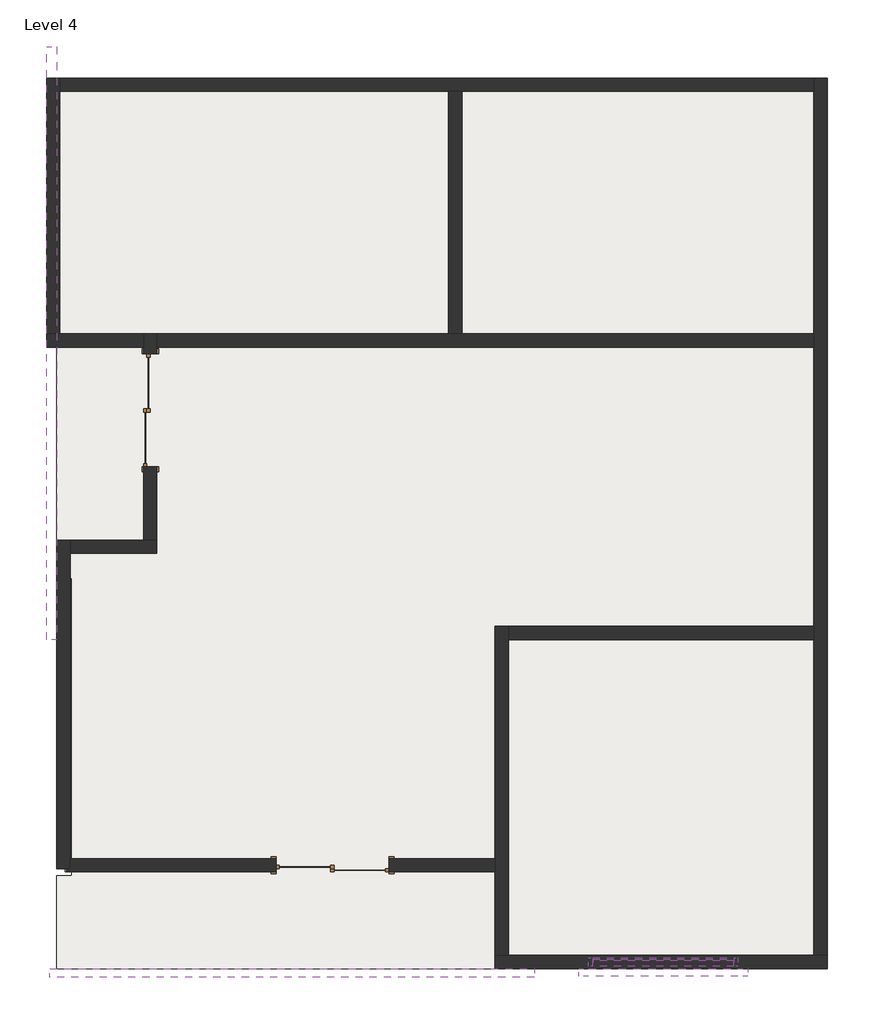
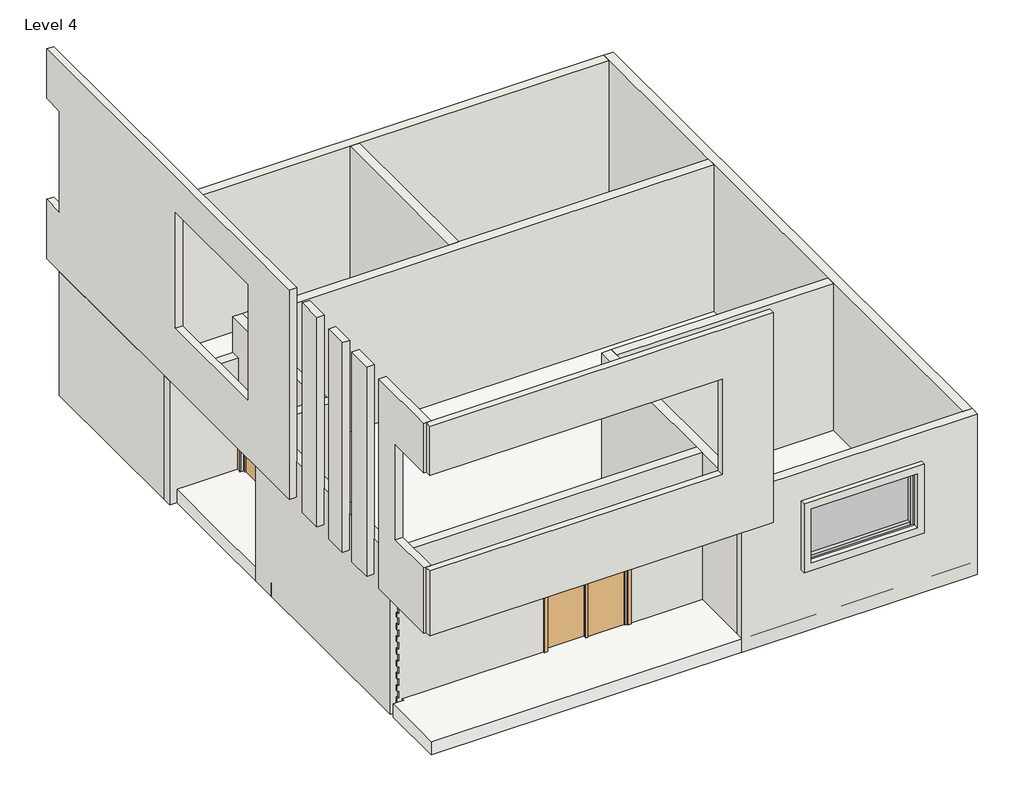
# One storey: 16 walls, 4 members, 2 doors, 1 plate, 1 roof.
"""IFC4 building model written with IfcOpenShell, lengths in millimetres."""

from ifc_helpers import new_model, si_unit, frame, origin, place, context, project, spatial, polyline, outline, extrude, faceted_brep, transform, mapped, element, save
from components import door_076b30e0, member_3a6679d5, member_c08f7e50, system_panel_glazed_5a0db22b, walls_2_walls_1_3aef9765, walls_7_walls_7_28da2d4c, walls_8_walls_8_57d20523

model = new_model("IFC4")

# Units and contexts
model_context = context("Model", 3, world=origin())
ifc_project = project(units=[si_unit("LENGTHUNIT", "METRE", prefix="MILLI")], contexts=[model_context])

# Site, building, storey
site = spatial("IfcSite", under=ifc_project)
building = spatial("IfcBuilding", under=site)
storey = spatial("IfcBuildingStorey", under=building, Name="Level 4", Elevation=10972.8)

# Doors
placement = place(None, origin())
door_shape = door_076b30e0(model_context)
element("IfcDoor", 1, ObjectType="Door-Double-Sliding : 68\" x 80\"", at=placement, inside=storey, context=model_context, shape_type="MappedRepresentation", body=[
    mapped(door_shape, transform((-7304.8227738, 4545.1674246, 11074.4), x_axis=(0.0, 1.0, 0.0), y_axis=(-1.0, 0.0, 0.0), z_axis=(0.0, 0.0, 1.0))),
])
element("IfcDoor", 2, ObjectType="Door-Double-Sliding : 68\" x 80\"", at=placement, inside=storey, context=model_context, shape_type="MappedRepresentation", body=[
    mapped(door_shape, transform((-4644.5436544, -2281.0825754, 11176.0), x_axis=(-1.0, 0.0, 0.0), y_axis=(0.0, -1.0, 0.0), z_axis=(0.0, 0.0, 1.0))),
])

# Members
member_shape = member_3a6679d5(model_context)
element("IfcMember", 3, ObjectType="Rectangular Mullion : 2.5\" x 5\" rectangular", at=placement, inside=storey, context=model_context, shape_type="MappedRepresentation", body=[
    mapped(member_shape, transform((1560.0533085, -3887.6325754, 12576.3422066), x_axis=(1.0, 0.0, 0.0), y_axis=(0.0, -1.0, 0.0), z_axis=(0.0, 0.0, -1.0))),
])
member_2_shape = member_c08f7e50(model_context)
element("IfcMember", 4, ObjectType="Rectangular Mullion : 2.5\" x 5\" rectangular", at=placement, inside=storey, context=model_context, shape_type="MappedRepresentation", body=[
    mapped(member_2_shape, transform((-662.4466915, -3887.6325754, 12576.3422066), x_axis=(0.0, 0.0, -1.0), y_axis=(0.0, -1.0, 0.0), z_axis=(-1.0, 0.0, 0.0))),
])
element("IfcMember", 5, ObjectType="Rectangular Mullion : 2.5\" x 5\" rectangular", at=placement, inside=storey, context=model_context, shape_type="MappedRepresentation", body=[
    mapped(member_2_shape, transform((1496.5533085, -3887.6325754, 13807.224337), x_axis=(0.0, 0.0, 1.0), y_axis=(0.0, -1.0, 0.0), z_axis=(1.0, 0.0, 0.0))),
])
element("IfcMember", 6, ObjectType="Rectangular Mullion : 2.5\" x 5\" rectangular", at=placement, inside=storey, context=model_context, shape_type="MappedRepresentation", body=[
    mapped(member_shape, transform((-725.9466915, -3887.6325754, 13807.224337), x_axis=(-1.0, 0.0, 0.0), y_axis=(0.0, -1.0, 0.0), z_axis=(0.0, 0.0, 1.0))),
])

# Plate
system_panel_glazed_shape = system_panel_glazed_5a0db22b(model_context)
element("IfcPlate", 7, ObjectType="System Panel : Glazed", at=placement, inside=storey, context=model_context, shape_type="MappedRepresentation", body=[
    mapped(system_panel_glazed_shape, transform((417.0533085, -3887.6325754, 12639.8422066), x_axis=(1.0, 0.0, 0.0), y_axis=(0.0, 1.0, 0.0), z_axis=(0.0, 0.0, 1.0))),
])

# Roof
element("IfcRoof", 8, ObjectType="Generic - 12\"", at=placement, inside=storey, context=model_context, shape_type="SweptSolid", body=[
    extrude(outline(polyline([(-8860.5727738, 9472.7674246), (2924.6563456, 9472.7674246), (2924.6563456, -3989.2325754), (-8860.5727738, -3989.2325754), (-8860.5727738, -2566.8325754), (-8631.9727738, -2566.8325754), (-8631.9727738, 1979.7674246), (-8860.5727738, 1979.7674246), (-8860.5727738, 9472.7674246)])), frame((0.0, 0.0, 10972.8), z_axis=(0.0, 0.0, 1.0), x_axis=(1.0, 0.0, 0.0)), (0.0, 0.0, 1.0), 304.8),
])

# Walls
element("IfcWall", 9, ObjectType="Generic - 8\"", at=placement, inside=storey, context=model_context, shape_type="Brep", body=[
    faceted_brep([(2924.6563456, -3786.0325754, 10972.8), (2721.4563456, -3786.0325754, 10972.8), (-1952.1436544, -3786.0325754, 10972.8), (-2155.3436544, -3786.0325754, 10972.8), (-2155.3436544, -3786.0325754, 14630.4), (-1952.1436544, -3786.0325754, 14630.4), (2721.4563456, -3786.0325754, 14630.4), (2924.6563456, -3786.0325754, 14630.4), (1560.0533085, -3786.0325754, 13807.224337), (-725.9466915, -3786.0325754, 13807.224337), (-725.9466915, -3786.0325754, 12576.3422066), (1560.0533085, -3786.0325754, 12576.3422066), (2924.6563456, -3989.2325754, 10972.8), (2924.6563456, -3989.2325754, 14630.4), (-2155.3436544, -3989.2325754, 14630.4), (-2155.3436544, -3989.2325754, 10972.8), (1560.0533085, -3989.2325754, 13807.224337), (1560.0533085, -3989.2325754, 12576.3422066), (-725.9466915, -3989.2325754, 12576.3422066), (-725.9466915, -3989.2325754, 13807.224337)], [[[0, 1, 2, 3, 4, 5, 6, 7], [8, 9, 10, 11]], [[12, 13, 14, 15], [16, 17, 18, 19]], [[4, 3, 15, 14]], [[0, 7, 13, 12]], [[3, 2, 1, 0, 12, 15]], [[7, 6, 5, 4, 14, 13]], [[9, 8, 16, 19]], [[10, 9, 19, 18]], [[11, 10, 18, 17]], [[8, 11, 17, 16]]]),
])
element("IfcWall", 10, ObjectType="Generic - 8\"", at=placement, inside=storey, context=model_context, shape_type="Brep", body=[
    faceted_brep([(-1952.1436544, -3786.0325754, 10972.8), (-1952.1436544, 1039.9674246, 10972.8), (-1952.1436544, 1243.1674246, 10972.8), (-1952.1436544, 1243.1674246, 14630.4), (-1952.1436544, 1039.9674246, 14630.4), (-1952.1436544, -3786.0325754, 14630.4), (-2155.3436544, -3786.0325754, 10972.8), (-2155.3436544, -3786.0325754, 14630.4), (-2155.3436544, -2509.6825754, 14630.4), (-2155.3436544, -2306.4825754, 14630.4), (-2155.3436544, 1243.1674246, 14630.4), (-2155.3436544, 1243.1674246, 10972.8), (-2155.3436544, -2306.4825754, 10972.8), (-2155.3436544, -2509.6825754, 10972.8)], [[[0, 1, 2, 3, 4, 5]], [[6, 7, 8, 9, 10, 11, 12, 13]], [[2, 1, 0, 6, 13, 12, 11]], [[5, 4, 3, 10, 9, 8, 7]], [[0, 5, 7, 6]], [[3, 2, 11, 10]]]),
])
element("IfcWall", 11, ObjectType="Generic - 8\"", at=placement, inside=storey, context=model_context, shape_type="SweptSolid", body=[
    extrude(outline(polyline([(2716.475018, 1039.9674246), (-1952.1436544, 1039.9674246), (-1952.1436544, 1243.1674246), (2716.475018, 1243.1674246), (2716.475018, 1039.9674246)])), frame((0.0, 0.0, 10972.8), z_axis=(0.0, 0.0, 1.0), x_axis=(1.0, 0.0, 0.0)), (0.0, 0.0, 1.0), 3657.6),
])
element("IfcWall", 12, ObjectType="Generic - 8\"", at=placement, inside=storey, context=model_context, shape_type="SweptSolid", body=[
    extrude(outline(polyline([(2924.6563456, 9625.1674246), (2924.6563456, -3786.0325754), (2721.4563456, -3786.0325754), (2721.4563456, 9625.1674246), (2924.6563456, 9625.1674246)])), frame((0.0, 0.0, 10972.8), z_axis=(0.0, 0.0, 1.0), x_axis=(1.0, 0.0, 0.0)), (0.0, 0.0, 1.0), 3657.6),
])
element("IfcWall", 13, ObjectType="Generic - 8\"", at=placement, inside=storey, context=model_context, shape_type="Brep", body=[
    faceted_brep([(-8657.3727738, -2465.2325754, 10972.8), (-8657.3727738, -2306.4825754, 10972.8), (-8657.3727738, 2360.7674246, 10972.8), (-8657.3727738, 2563.9674246, 10972.8), (-8657.3727738, 2563.9674246, 14630.4), (-8657.3727738, 2360.7674246, 14630.4), (-8657.3727738, -2306.4825754, 14630.4), (-8657.3727738, -2465.2325754, 14630.4), (-8860.5727738, -2465.2325754, 10972.8), (-8860.5727738, -2465.2325754, 11328.4), (-8860.5727738, -2465.2325754, 11480.8), (-8860.5727738, -2465.2325754, 11607.8), (-8860.5727738, -2465.2325754, 11760.2), (-8860.5727738, -2465.2325754, 11887.2), (-8860.5727738, -2465.2325754, 12039.6), (-8860.5727738, -2465.2325754, 12166.6), (-8860.5727738, -2465.2325754, 12319.0), (-8860.5727738, -2465.2325754, 12446.0), (-8860.5727738, -2465.2325754, 12598.4), (-8860.5727738, -2465.2325754, 12725.4), (-8860.5727738, -2465.2325754, 12877.8), (-8860.5727738, -2465.2325754, 13004.8), (-8860.5727738, -2465.2325754, 13157.2), (-8860.5727738, -2465.2325754, 13258.8), (-8860.5727738, -2465.2325754, 13411.2), (-8860.5727738, -2465.2325754, 13563.6), (-8860.5727738, -2465.2325754, 13716.0), (-8860.5727738, -2465.2325754, 14630.4), (-8860.5727738, 2563.9674246, 14630.4), (-8860.5727738, 2563.9674246, 10972.8), (-8733.5727738, -2465.2325754, 10972.8), (-8733.5727738, -2465.2325754, 14630.4)], [[[0, 1, 2, 3, 4, 5, 6, 7]], [[8, 9, 10, 11, 12, 13, 14, 15, 16, 17, 18, 19, 20, 21, 22, 23, 24, 25, 26, 27, 28, 29]], [[3, 2, 1, 0, 30, 8, 29]], [[7, 6, 5, 4, 28, 27, 31]], [[0, 7, 31, 27, 26, 25, 24, 23, 22, 21, 20, 19, 18, 17, 16, 15, 14, 13, 12, 11, 10, 9, 8, 30]], [[4, 3, 29, 28]]]),
])
element("IfcWall", 14, ObjectType="Generic - 8\"", at=placement, inside=storey, context=model_context, shape_type="Brep", body=[
    faceted_brep([(-8657.3727738, 2360.7674246, 10972.8), (-7330.2227738, 2360.7674246, 10972.8), (-7330.2227738, 2360.7674246, 14630.4), (-8657.3727738, 2360.7674246, 14630.4), (-8657.3727738, 2563.9674246, 10972.8), (-8657.3727738, 2563.9674246, 14630.4), (-7533.4227738, 2563.9674246, 14630.4), (-7330.2227738, 2563.9674246, 14630.4), (-7330.2227738, 2563.9674246, 10972.8), (-7533.4227738, 2563.9674246, 10972.8)], [[[0, 1, 2, 3]], [[4, 5, 6, 7, 8, 9]], [[1, 0, 4, 9, 8]], [[3, 2, 7, 6, 5]], [[0, 3, 5, 4]], [[2, 1, 8, 7]]]),
])
element("IfcWall", 15, ObjectType="Generic - 8\"", at=placement, inside=storey, context=model_context, shape_type="Brep", body=[
    faceted_brep([(-7330.2227738, 2563.9674246, 10972.8), (-7330.2227738, 5510.3674246, 10972.8), (-7330.2227738, 5713.5674246, 10972.8), (-7330.2227738, 5713.5674246, 14630.4), (-7330.2227738, 5510.3674246, 14630.4), (-7330.2227738, 2563.9674246, 14630.4), (-7330.2227738, 3681.5674246, 13106.4), (-7330.2227738, 5408.7674246, 13106.4), (-7330.2227738, 5408.7674246, 11074.4), (-7330.2227738, 3681.5674246, 11074.4), (-7533.4227738, 2563.9674246, 10972.8), (-7533.4227738, 2563.9674246, 14630.4), (-7533.4227738, 5713.5674246, 14630.4), (-7533.4227738, 5713.5674246, 13807.224337), (-7533.4227738, 5713.5674246, 10972.8), (-7533.4227738, 5510.3674246, 10972.8), (-7533.4227738, 3681.5674246, 13106.4), (-7533.4227738, 3681.5674246, 11074.4), (-7533.4227738, 5408.7674246, 11074.4), (-7533.4227738, 5408.7674246, 13106.4)], [[[0, 1, 2, 3, 4, 5], [6, 7, 8, 9]], [[10, 11, 12, 13, 14, 15], [16, 17, 18, 19]], [[2, 1, 0, 10, 15, 14]], [[5, 4, 3, 12, 11]], [[0, 5, 11, 10]], [[17, 16, 6, 9]], [[18, 17, 9, 8]], [[19, 18, 8, 7]], [[16, 19, 7, 6]], [[2, 14, 13, 12, 3]]]),
])
element("IfcWall", 16, ObjectType="Generic - 8\"", at=placement, inside=storey, context=model_context, shape_type="Brep", body=[
    faceted_brep([(-7533.4227738, 5713.5674246, 10972.8), (-8815.124982, 5713.5674246, 10972.8), (-9018.324982, 5713.5674246, 10972.8), (-9018.324982, 5713.5674246, 13807.224337), (-8815.124982, 5713.5674246, 13807.224337), (-7533.4227738, 5713.5674246, 13807.224337), (-7533.4227738, 5510.3674246, 10972.8), (-7533.4227738, 5510.3674246, 13807.224337), (-9018.324982, 5510.3674246, 13807.224337), (-9018.324982, 5510.3674246, 10972.8)], [[[0, 1, 2, 3, 4, 5]], [[6, 7, 8, 9]], [[2, 1, 0, 6, 9]], [[5, 4, 3, 8, 7]], [[0, 5, 7, 6]], [[3, 2, 9, 8]]]),
])
element("IfcWall", 17, ObjectType="Generic - 8\"", at=placement, inside=storey, context=model_context, shape_type="Brep", body=[
    faceted_brep([(-8815.124982, 5713.5674246, 10972.8), (-8815.124982, 9421.9674246, 10972.8), (-8815.124982, 9625.1674246, 10972.8), (-8815.124982, 9625.1674246, 13807.224337), (-8815.124982, 5713.5674246, 13807.224337), (-9018.324982, 5713.5674246, 10972.8), (-9018.324982, 5713.5674246, 13807.224337), (-9018.324982, 9625.1674246, 13807.224337), (-9018.324982, 9625.1674246, 10972.8)], [[[0, 1, 2, 3, 4]], [[5, 6, 7, 8]], [[2, 1, 0, 5, 8]], [[4, 3, 7, 6]], [[0, 4, 6, 5]], [[3, 2, 8, 7]]]),
])
element("IfcWall", 18, ObjectType="Generic - 8\"", at=placement, inside=storey, context=model_context, shape_type="Brep", body=[
    faceted_brep([(-8815.124982, 9421.9674246, 10972.8), (-2866.5436544, 9421.9674246, 10972.8), (-2663.3436544, 9421.9674246, 10972.8), (2716.475018, 9421.9674246, 10972.8), (2716.475018, 9421.9674246, 14630.4), (-2663.3436544, 9421.9674246, 14630.4), (-2866.5436544, 9421.9674246, 14630.4), (-8815.124982, 9421.9674246, 14630.4), (-8815.124982, 9625.1674246, 10972.8), (-8815.124982, 9625.1674246, 13807.224337), (-8815.124982, 9625.1674246, 14630.4), (2716.475018, 9625.1674246, 14630.4), (2716.475018, 9625.1674246, 10972.8)], [[[0, 1, 2, 3, 4, 5, 6, 7]], [[8, 9, 10, 11, 12]], [[3, 2, 1, 0, 8, 12]], [[4, 3, 12, 11]], [[7, 6, 5, 4, 11, 10]], [[0, 7, 10, 9, 8]]]),
])
element("IfcWall", 19, ObjectType="Generic - 8\"", at=placement, inside=storey, context=model_context, shape_type="Brep", body=[
    faceted_brep([(-7330.2227738, 5510.3674246, 10972.8), (2716.475018, 5510.3674246, 10972.8), (2716.475018, 5510.3674246, 14630.4), (-7330.2227738, 5510.3674246, 14630.4), (-7330.2227738, 5713.5674246, 10972.8), (-7330.2227738, 5713.5674246, 14630.4), (-2866.5436544, 5713.5674246, 14630.4), (-2663.3436544, 5713.5674246, 14630.4), (2716.475018, 5713.5674246, 14630.4), (2716.475018, 5713.5674246, 10972.8), (-2663.3436544, 5713.5674246, 10972.8), (-2866.5436544, 5713.5674246, 10972.8)], [[[0, 1, 2, 3]], [[4, 5, 6, 7, 8, 9, 10, 11]], [[1, 0, 4, 11, 10, 9]], [[2, 1, 9, 8]], [[3, 2, 8, 7, 6, 5]], [[0, 3, 5, 4]]]),
])
element("IfcWall", 20, ObjectType="Generic - 8\"", at=placement, inside=storey, context=model_context, shape_type="SweptSolid", body=[
    extrude(outline(polyline([(-2663.3436544, 9421.9674246), (-2663.3436544, 5713.5674246), (-2866.5436544, 5713.5674246), (-2866.5436544, 9421.9674246), (-2663.3436544, 9421.9674246)])), frame((0.0, 0.0, 10972.8), z_axis=(0.0, 0.0, 1.0), x_axis=(1.0, 0.0, 0.0)), (0.0, 0.0, 1.0), 3657.6),
])
element("IfcWall", 21, ObjectType="Generic - 8\"", at=placement, inside=storey, context=model_context, shape_type="Brep", body=[
    faceted_brep([(-8733.5727738, -2509.6825754, 10972.8), (-2155.3436544, -2509.6825754, 10972.8), (-2155.3436544, -2509.6825754, 14630.4), (-8733.5727738, -2509.6825754, 14630.4), (-8733.5727738, -2509.6825754, 13716.0), (-8708.1727738, -2509.6825754, 13716.0), (-8708.1727738, -2509.6825754, 13563.6), (-8733.5727738, -2509.6825754, 13563.6), (-8733.5727738, -2509.6825754, 13411.2), (-8708.1727738, -2509.6825754, 13411.2), (-8708.1727738, -2509.6825754, 13258.8), (-8733.5727738, -2509.6825754, 13258.8), (-8733.5727738, -2509.6825754, 13157.2), (-8708.1727738, -2509.6825754, 13157.2), (-8708.1727738, -2509.6825754, 13004.8), (-8733.5727738, -2509.6825754, 13004.8), (-8733.5727738, -2509.6825754, 12877.8), (-8708.1727738, -2509.6825754, 12877.8), (-8708.1727738, -2509.6825754, 12725.4), (-8733.5727738, -2509.6825754, 12725.4), (-8733.5727738, -2509.6825754, 12598.4), (-8708.1727738, -2509.6825754, 12598.4), (-8708.1727738, -2509.6825754, 12446.0), (-8733.5727738, -2509.6825754, 12446.0), (-8733.5727738, -2509.6825754, 12319.0), (-8708.1727738, -2509.6825754, 12319.0), (-8708.1727738, -2509.6825754, 12166.6), (-8733.5727738, -2509.6825754, 12166.6), (-8733.5727738, -2509.6825754, 12039.6), (-8708.1727738, -2509.6825754, 12039.6), (-8708.1727738, -2509.6825754, 11887.2), (-8733.5727738, -2509.6825754, 11887.2), (-8733.5727738, -2509.6825754, 11760.2), (-8708.1727738, -2509.6825754, 11760.2), (-8708.1727738, -2509.6825754, 11607.8), (-8733.5727738, -2509.6825754, 11607.8), (-8733.5727738, -2509.6825754, 11480.8), (-8708.1727738, -2509.6825754, 11480.8), (-8708.1727738, -2509.6825754, 11328.4), (-8733.5727738, -2509.6825754, 11328.4), (-3780.9436544, -2509.6825754, 13208.0), (-3780.9436544, -2509.6825754, 11176.0), (-5508.1436544, -2509.6825754, 11176.0), (-5508.1436544, -2509.6825754, 13208.0), (-2155.3436544, -2306.4825754, 10972.8), (-8657.3727738, -2306.4825754, 10972.8), (-8657.3727738, -2306.4825754, 14630.4), (-2155.3436544, -2306.4825754, 14630.4), (-3780.9436544, -2306.4825754, 11176.0), (-3780.9436544, -2306.4825754, 13208.0), (-5508.1436544, -2306.4825754, 13208.0), (-5508.1436544, -2306.4825754, 11176.0), (-8733.5727738, -2465.2325754, 10972.8), (-8657.3727738, -2465.2325754, 10972.8), (-8657.3727738, -2465.2325754, 14630.4), (-8733.5727738, -2465.2325754, 14630.4), (-8733.5727738, -2465.2325754, 13716.0), (-8733.5727738, -2465.2325754, 11328.4), (-8733.5727738, -2465.2325754, 11480.8), (-8733.5727738, -2465.2325754, 11607.8), (-8733.5727738, -2465.2325754, 11760.2), (-8733.5727738, -2465.2325754, 11887.2), (-8733.5727738, -2465.2325754, 12039.6), (-8733.5727738, -2465.2325754, 12166.6), (-8733.5727738, -2465.2325754, 12319.0), (-8733.5727738, -2465.2325754, 12446.0), (-8733.5727738, -2465.2325754, 12598.4), (-8733.5727738, -2465.2325754, 12725.4), (-8733.5727738, -2465.2325754, 12877.8), (-8733.5727738, -2465.2325754, 13004.8), (-8733.5727738, -2465.2325754, 13157.2), (-8733.5727738, -2465.2325754, 13258.8), (-8733.5727738, -2465.2325754, 13411.2), (-8733.5727738, -2465.2325754, 13563.6), (-8708.1727738, -2465.2325754, 11328.4), (-8708.1727738, -2465.2325754, 11480.8), (-8708.1727738, -2465.2325754, 11607.8), (-8708.1727738, -2465.2325754, 11760.2), (-8708.1727738, -2465.2325754, 11887.2), (-8708.1727738, -2465.2325754, 12039.6), (-8708.1727738, -2465.2325754, 12166.6), (-8708.1727738, -2465.2325754, 12319.0), (-8708.1727738, -2465.2325754, 12446.0), (-8708.1727738, -2465.2325754, 12598.4), (-8708.1727738, -2465.2325754, 12725.4), (-8708.1727738, -2465.2325754, 12877.8), (-8708.1727738, -2465.2325754, 13004.8), (-8708.1727738, -2465.2325754, 13157.2), (-8708.1727738, -2465.2325754, 13258.8), (-8708.1727738, -2465.2325754, 13411.2), (-8708.1727738, -2465.2325754, 13563.6), (-8708.1727738, -2465.2325754, 13716.0)], [[[0, 1, 2, 3, 4, 5, 6, 7, 8, 9, 10, 11, 12, 13, 14, 15, 16, 17, 18, 19, 20, 21, 22, 23, 24, 25, 26, 27, 28, 29, 30, 31, 32, 33, 34, 35, 36, 37, 38, 39], [40, 41, 42, 43]], [[44, 45, 46, 47], [48, 49, 50, 51]], [[1, 0, 52, 53, 45, 44]], [[3, 2, 47, 46, 54, 55]], [[2, 1, 44, 47]], [[3, 55, 56, 4]], [[52, 0, 39, 57]], [[58, 36, 35, 59]], [[60, 32, 31, 61]], [[62, 28, 27, 63]], [[64, 24, 23, 65]], [[66, 20, 19, 67]], [[68, 16, 15, 69]], [[70, 12, 11, 71]], [[72, 8, 7, 73]], [[55, 54, 53, 52, 57, 74, 75, 58, 59, 76, 77, 60, 61, 78, 79, 62, 63, 80, 81, 64, 65, 82, 83, 66, 67, 84, 85, 68, 69, 86, 87, 70, 71, 88, 89, 72, 73, 90, 91, 56]], [[46, 45, 53, 54]], [[75, 37, 36, 58]], [[37, 75, 74, 38]], [[38, 74, 57, 39]], [[77, 33, 32, 60]], [[33, 77, 76, 34]], [[34, 76, 59, 35]], [[79, 29, 28, 62]], [[29, 79, 78, 30]], [[30, 78, 61, 31]], [[81, 25, 24, 64]], [[25, 81, 80, 26]], [[26, 80, 63, 27]], [[83, 21, 20, 66]], [[21, 83, 82, 22]], [[22, 82, 65, 23]], [[85, 17, 16, 68]], [[17, 85, 84, 18]], [[18, 84, 67, 19]], [[87, 13, 12, 70]], [[13, 87, 86, 14]], [[14, 86, 69, 15]], [[89, 9, 8, 72]], [[9, 89, 88, 10]], [[10, 88, 71, 11]], [[91, 5, 4, 56]], [[5, 91, 90, 6]], [[6, 90, 73, 7]], [[41, 40, 49, 48]], [[42, 41, 48, 51]], [[43, 42, 51, 50]], [[40, 43, 50, 49]]]),
])
walls_2_walls_1_shape = walls_2_walls_1_3aef9765(model_context)
element("IfcWall", 22, ObjectType="Walls 2 : Walls 1", at=placement, inside=storey, context=model_context, shape_type="MappedRepresentation", body=[
    mapped(walls_2_walls_1_shape, transform((0.0, 0.0, 0.0), x_axis=(1.0, 0.0, 0.0), y_axis=(0.0, 1.0, 0.0), z_axis=(0.0, 0.0, 1.0))),
])
walls_7_walls_7_shape = walls_7_walls_7_28da2d4c(model_context)
element("IfcWall", 23, ObjectType="Walls 7 : Walls 7", at=placement, inside=storey, context=model_context, shape_type="MappedRepresentation", body=[
    mapped(walls_7_walls_7_shape, transform((0.0, 0.0, 0.0), x_axis=(1.0, 0.0, 0.0), y_axis=(0.0, 1.0, 0.0), z_axis=(0.0, 0.0, 1.0))),
])
walls_8_walls_8_shape = walls_8_walls_8_57d20523(model_context)
element("IfcWall", 24, ObjectType="Walls 8 : Walls 8", at=placement, inside=storey, context=model_context, shape_type="MappedRepresentation", body=[
    mapped(walls_8_walls_8_shape, transform((0.0, 0.0, 0.0), x_axis=(1.0, 0.0, 0.0), y_axis=(0.0, 1.0, 0.0), z_axis=(0.0, 0.0, 1.0))),
])

save(model, "model.ifc")

# Revit data of these elements
# Type "Door-Double-Sliding : 68\" x 80\""
#   Type Mark = "10"
#   Construction Type Id = "opn-d45"
#   Assembly Code = "C1020"
#   Analytic Construction = "Wood frame, double glass door "
#   Thickness = 0' - 2"
#   Thermal Resistance (R) = 1.8150 (h·ft²·°F)/BTU
#   Heat Transfer Coefficient (U) = 0.5510 BTU/(h·ft²·°F)
#   Height = 6' - 8"
#   Rail Width = 0' - 2"
#   Stiles = 0' - 2"
#   Trim Projection Ext = 0' - 1"
#   Trim Projection Int = 0' - 1"
#   Trim Width = 0' - 3"
#   Width = 5' - 8"
#   Define Thermal Properties by = 1
#   Glazing = Glass
#   Panel Material = Wood - Birch - Solid Stained Light Low Gloss
#   Trim Material = Paint - Sienna
#   Visual Light Transmittance = 0
#   Solar Heat Gain Coefficient = 0
#   Function = (empty or 0)
#   Wall Closure = (empty or 0)
# Type "Rectangular Mullion : 2.5\" x 5\" rectangular"
#   built-in parameter 1007304 = 0.416667 (stored number, unit not read)
#   built-in parameter 1007301 = 0.104167 (stored number, unit not read)
#   built-in parameter 1007300 = 0.104167 (stored number, unit not read)
# Type "System Panel : Glazed"
#   Construction Type Id = "GSP4R"
#   Analytic Construction = "1/8 in Pilkington single glazing"
#   Visual Light Transmittance = 0.9
#   Solar Heat Gain Coefficient = 0.86
#   Heat Transfer Coefficient (U) = 1.18115 BTU/(h·ft²·°F)
# Type "Generic - 12\""
#   Assembly Code = "B1020"
#   Layers, outside or top first: 1' - 0" no material (function 1)
# Type "Generic - 8\""
#   Assembly Code = "B2010"
#   Layers, outside or top first: 0' - 8" no material (function 1)
# Elements 1, 2 (IfcDoor, "Door-Double-Sliding : 68\" x 80\"")
#   Phase Created = New Construction
#   Materials on its faces: "Paint - Sienna", "Wood - Birch - Solid Stained Light Low Gloss", "Glass"
# Elements 3, 4, 5, 6 (IfcMember, "Rectangular Mullion : 2.5\" x 5\" rectangular")
#   Phase Created = New Construction
#   Materials on its faces: "Aluminum"
# Element 7 (IfcPlate, "System Panel : Glazed")
#   Phase Created = New Construction
#   Materials on its faces: "Glass"
# Element 8 (IfcRoof, "Generic - 12\"")
#   built-in parameter 1001705 = 37 (stored number, unit not read)
#   built-in parameter 1001710 = 33615
#   Phase Created = New Construction
#   Materials on its faces: "Default Roof"
# Elements 9, 10, 11, 12, 13, 14, 15, 18, 19, 20, 21 (IfcWall, "Generic - 8\"")
#   Top Offset = 0' - 0"
#   Base Offset = 0' - 0"
#   Unconnected Height = 12' - 0"
#   wall height = 12' - 0"
#   Phase Created = New Construction
#   Base Constraint = Level 4
#   Materials on its faces: "Default Wall"
# Elements 16, 17 (IfcWall, "Generic - 8\"")
#   Top Offset = 0' - 0"
#   Base Offset = 0' - 0"
#   Unconnected Height = 9' - 3.59151"
#   wall height = 9' - 3.59151"
#   Phase Created = New Construction
#   Base Constraint = Level 4
#   Materials on its faces: "Default Wall"
# Element 22 (IfcWall, "Walls 2 : Walls 1")
#   Phase Created = New Construction
#   Materials on its faces: "Default Wall"
# Element 23 (IfcWall, "Walls 7 : Walls 7")
#   Phase Created = New Construction
#   Materials on its faces: "Default Wall"
# Element 24 (IfcWall, "Walls 8 : Walls 8")
#   Phase Created = New Construction
#   Materials on its faces: "Default Wall"
# Materials
#   "Glass": class "Glass", colour RGB 0 128 192, transparency 0.75, Description = "Soda Lime Glass", Cost = 0
#   "Wood - Birch - Solid Stained Light Low Gloss": class "Wood", colour RGB 210 159 95, transparency 0, Cost = 0
#   "Paint - Sienna": colour RGB 118 70 51, transparency 0, Cost = 0
#   "Aluminum": class "Metal", colour RGB 247 247 247, transparency 0, Description = "Aluminum 6061", Cost = 0
#   "Default Roof": colour RGB 88 101 114, transparency 0
#   "Default Wall": colour RGB 128 128 128, transparency 0
